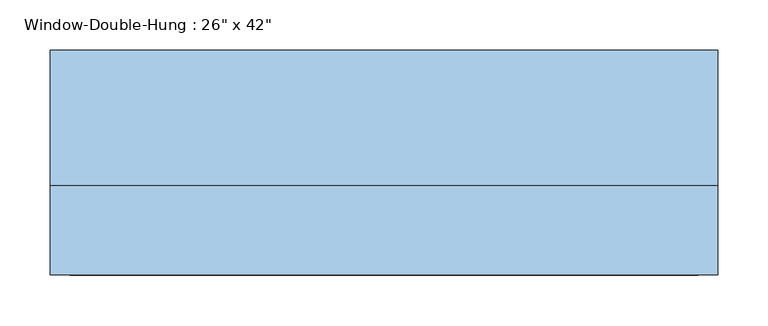
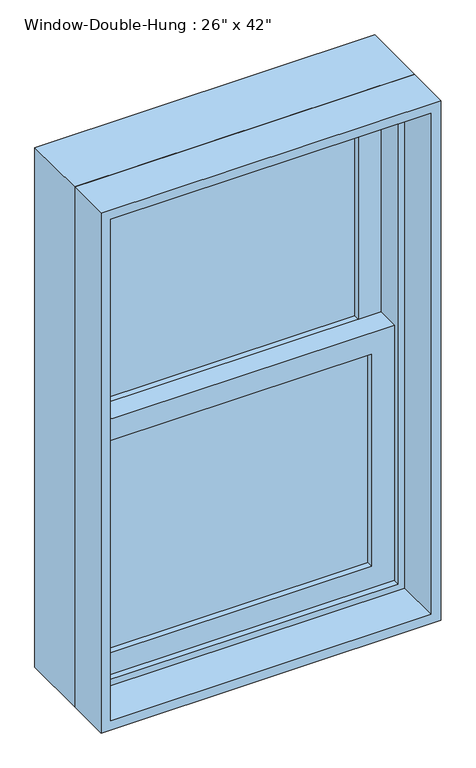
"""IFC4 building model written with IfcOpenShell, lengths in millimetres: window geometry."""

from ifc_helpers import new_model, si_unit, frame, origin, place, context, project, spatial, polyline, outline, extrude, source, transform, mapped, element, save


def window_8debb0fa(model_context):
    return source(origin(), model_context, "Body", "SweptSolid", [
        extrude(outline(polyline([(254.0, 31.75), (254.0, 25.4), (-254.0, 25.4), (-254.0, 31.75), (254.0, 31.75)])), frame((0.0, 0.0, 990.6), z_axis=(0.0, 0.0, 1.0), x_axis=(1.0, 0.0, 0.0)), (0.0, 0.0, 1.0), 434.975),
        extrude(outline(polyline([(-254.0, 19.05), (254.0, 19.05), (254.0, 12.7), (-254.0, 12.7), (-254.0, 19.05)])), frame((0.0, 0.0, 990.6), z_axis=(0.0, 0.0, 1.0), x_axis=(1.0, 0.0, 0.0)), (0.0, 0.0, 1.0), 434.975),
        extrude(outline(polyline([(254.0, 76.2), (254.0, 69.85), (-254.0, 69.85), (-254.0, 76.2), (254.0, 76.2)])), frame((0.0, 0.0, 1470.025), z_axis=(0.0, 0.0, 1.0), x_axis=(1.0, 0.0, 0.0)), (0.0, 0.0, 1.0), 434.975),
        extrude(outline(polyline([(-254.0, 63.5), (254.0, 63.5), (254.0, 57.15), (-254.0, 57.15), (-254.0, 63.5)])), frame((0.0, 0.0, 1470.025), z_axis=(0.0, 0.0, 1.0), x_axis=(1.0, 0.0, 0.0)), (0.0, 0.0, 1.0), 434.975),
        extrude(outline(polyline([(1470.025, -298.45), (946.15, -298.45), (946.15, 298.45), (1470.025, 298.45), (1470.025, -298.45)]), holes=[polyline([(1425.575, 254.0), (990.6, 254.0), (990.6, -254.0), (1425.575, -254.0), (1425.575, 254.0)])]), frame((0.0, 0.0, 0.0), z_axis=(0.0, 1.0, 0.0), x_axis=(0.0, 0.0, 1.0)), (0.0, 0.0, 1.0), 44.45),
        extrude(outline(polyline([(1949.45, -298.45), (1425.575, -298.45), (1425.575, 298.45), (1949.45, 298.45), (1949.45, -298.45)]), holes=[polyline([(1905.0, 254.0), (1470.025, 254.0), (1470.025, -254.0), (1905.0, -254.0), (1905.0, 254.0)])]), frame((0.0, 44.45, 0.0), z_axis=(0.0, 1.0, 0.0), x_axis=(0.0, 0.0, 1.0)), (0.0, 0.0, 1.0), 44.45),
        extrude(outline(polyline([(1981.2, -330.2), (914.4, -330.2), (914.4, 330.2), (1981.2, 330.2), (1981.2, -330.2)]), holes=[polyline([(1949.45, 298.45), (946.15, 298.45), (946.15, -298.45), (1949.45, -298.45), (1949.45, 298.45)])]), frame((0.0, -12.7, 0.0), z_axis=(0.0, 1.0, 0.0), x_axis=(0.0, 0.0, 1.0)), (0.0, 0.0, 1.0), 133.35),
        extrude(outline(polyline([(1981.2, 330.2), (1981.2, -330.2), (914.4, -330.2), (914.4, 330.2), (1981.2, 330.2)]), holes=[polyline([(1962.15, 311.15), (933.45, 311.15), (933.45, -311.15), (1962.15, -311.15), (1962.15, 311.15)])]), frame((0.0, -101.6, 0.0), z_axis=(0.0, 1.0, 0.0), x_axis=(0.0, 0.0, 1.0)), (0.0, 0.0, 1.0), 88.9),
    ])


if __name__ == "__main__":
    model = new_model("IFC4")
    model_context = context("Model", 3, world=origin())
    ifc_project = project(units=[si_unit("LENGTHUNIT", "METRE", prefix="MILLI")], contexts=[model_context])
    site = spatial("IfcSite", under=ifc_project)
    building = spatial("IfcBuilding", under=site)
    placement = place(None, origin())
    window_shape = window_8debb0fa(model_context)
    element("IfcWindow", 1, ObjectType="Window-Double-Hung : 26\" x 42\"", at=placement, inside=building, context=model_context, shape_type="MappedRepresentation", body=[
        mapped(window_shape, transform((0.0, 0.0, 0.0), x_axis=(1.0, 0.0, 0.0), y_axis=(0.0, 1.0, 0.0), z_axis=(0.0, 0.0, 1.0))),
    ])
    save(model, "model.ifc")

# Revit data of these elements
# Type "Window-Double-Hung : 26\" x 42\""
#   Type Mark = "11"
#   Fire Rating = "0.5h"
#   Construction Type Id = "DG-DR"
#   Assembly Code = "B2020100"
#   Analytic Construction = "Double glazing - domestic"
#   Wall Thickness [instance default] = 0' - 6"
#   Window Inset [instance default] = 0' - 0"
#   Visual Light Transmittance = 0.81
#   Thermal Resistance (R) = 1.8146 (h·ft²·°F)/BTU
#   Solar Heat Gain Coefficient = 0.76
#   Muntin Width = 1' - 8"
#   Muntin Height = 1' - 5 1/8"
#   Interior Wall Closure [instance default] = 0' - 1 1/2"
#   Rough Width = 2' - 2 1/2"
#   Rough Height = 3' - 6 1/2"
#   Frame Extension [instance default] = 0' - 1 1/4"
#   Exterior Wall Closure [instance default] = 0' - 0 1/2"
#   Extension Jamb [instance default] = 0' - 1 1/2"
#   Heat Transfer Coefficient (U) = 0.5511 BTU/(h·ft²·°F)
#   Height = 3' - 6"
#   Width = 2' - 2"
#   Define Thermal Properties by = 1
#   Top Muntin Visibility = yes
#   Indicator Visibility [instance default] = yes
#   Extension Jamb Visibility [instance default] = yes
#   Interior Trim Visibility [instance default] = yes
#   Exterior Trim Visibility [instance default] = yes
#   Define Thermal Properties by = 1
#   Bottom Muntin Visibility = yes
#   Muntin Pattern = Muntin Pattern_2x2 : Muntin Pattern_2x2
#   Interior Trim Material = Wood - Stained
#   Interior Trim = Trim-Window-Interior-Flat : Picture Frame
#   Exterior Trim Material = Clad - White
#   Exterior Trim = Trim-Window-Exterior-Flat : with Sill
#   Glass Panel Material = Glass
#   Exterior Frame Material = Clad - White
#   Interior Frame Material = Wood - Stained
#   Wall Closure = (empty or 0)
# Element 1 (IfcWindow, "Window-Double-Hung : 26\" x 42\"")
#   Wall Thickness = 0' - 8"
#   Extension Jamb = 0' - 3 1/2"
#   Materials on its faces: "Wood - Stained", "Glass", "Clad - White"
# Materials
#   "Wood - Stained": class "Wood", colour RGB 224 178 126, transparency 0, Cost = 0
#   "Clad - White": class "Wood", colour RGB 242 242 238, transparency 0, Cost = 0
#   "Glass": class "Glass", colour RGB 0 128 192, transparency 0.75, Description = "Soda Lime Glass", Cost = 0
